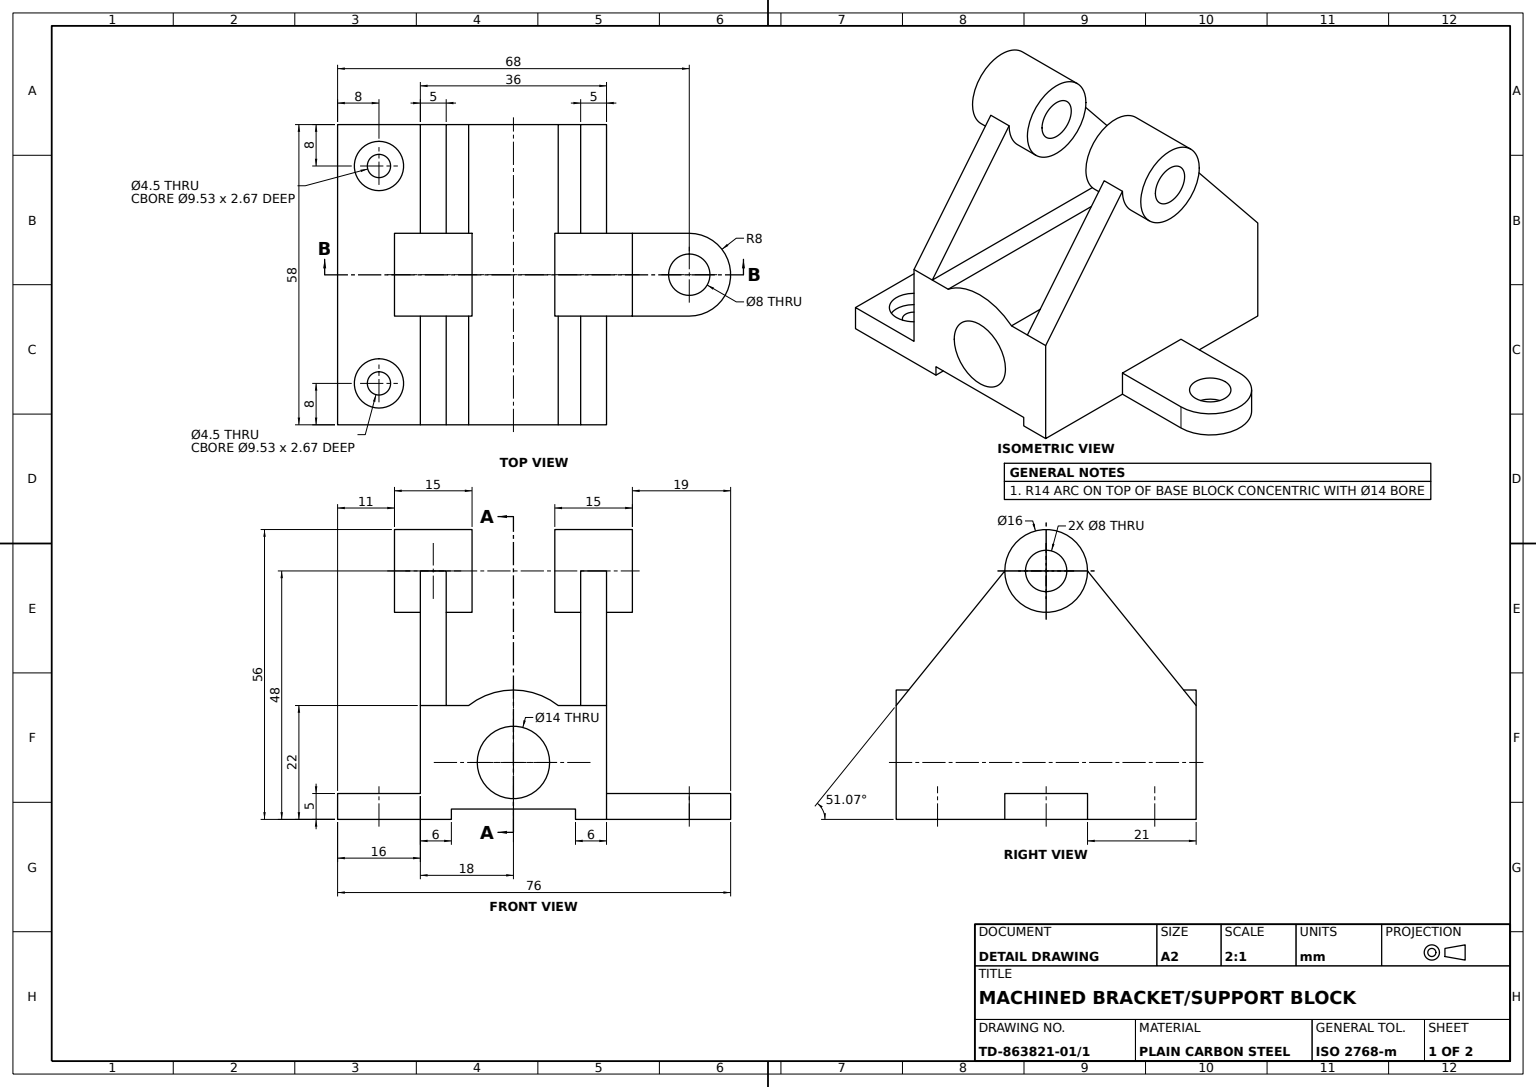
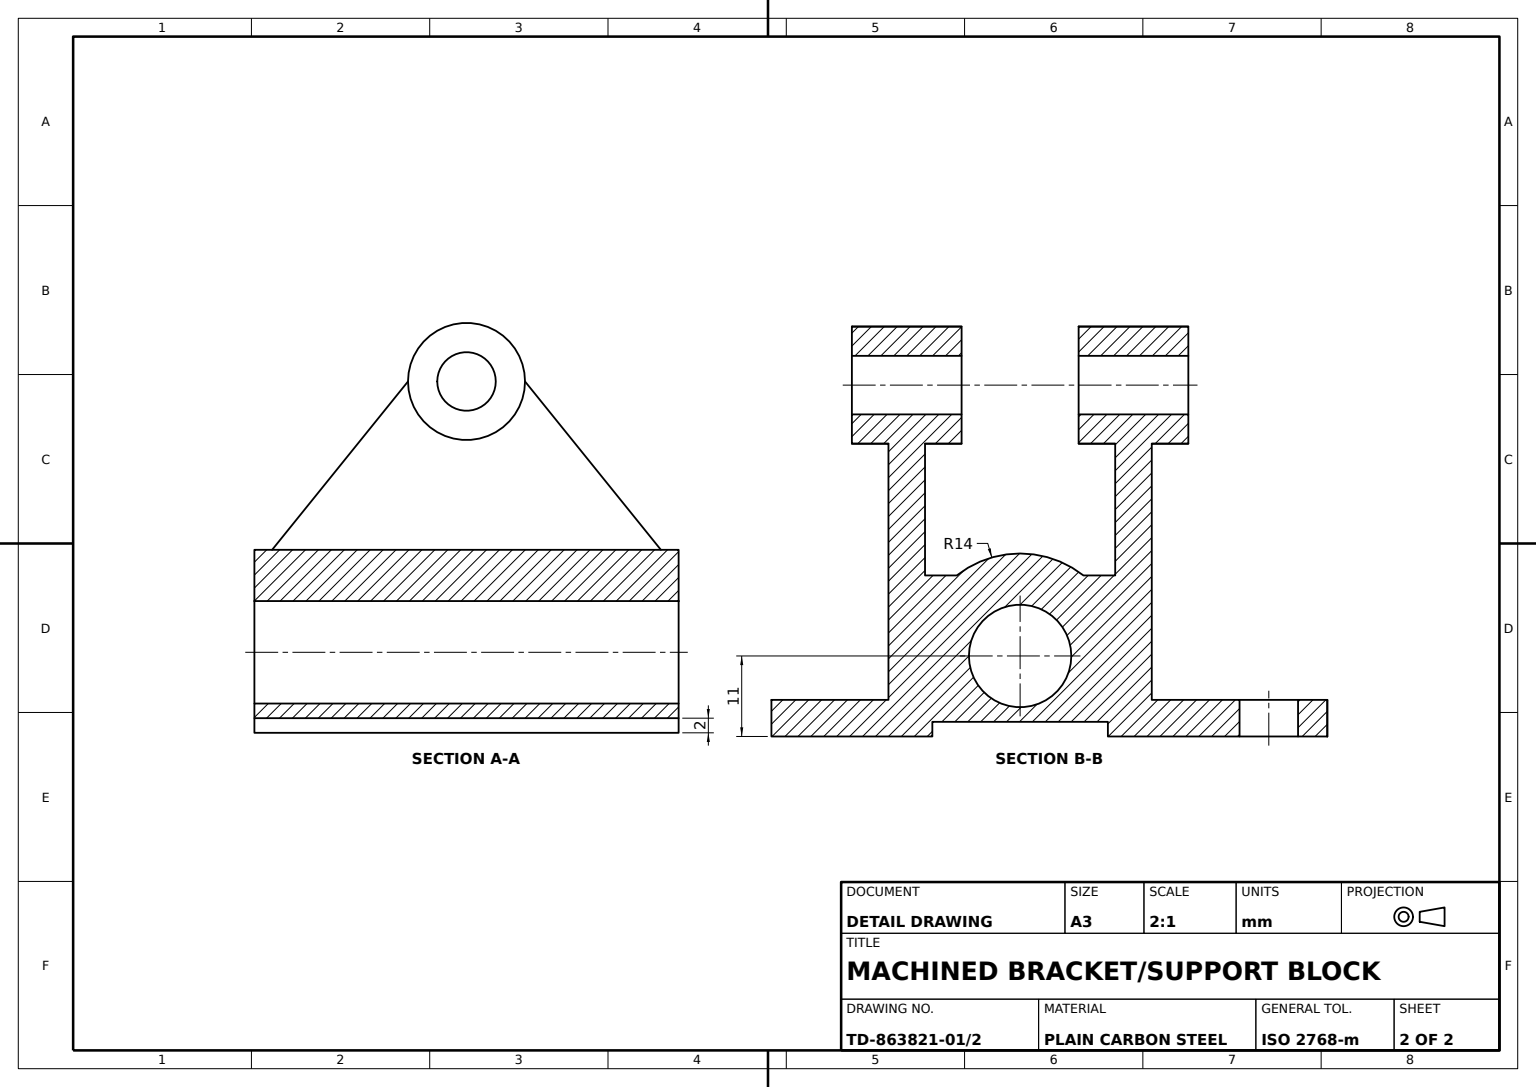
from build123d import *

# Parameters (mm, degrees)
BASE_BLOCK_DEPTH                = 58
FRONT_BORE_BOSS_DEPTH           = 58
FRONT_BORE_SKETCH_R             = 7
FRONT_BORE_DEPTH                = 73.698005475
LEFT_ARM_SKETCH_R               = 8
LEFT_ARM_SKETCH_R_2             = 4
LEFT_ARM_DEPTH                  = 5
LEFT_ARM_WEB_DEPTH              = 5
LEFT_START                      = 5
LEFT_PIVOT_BOSS_SKETCH_R        = 8
LEFT_PIVOT_BOSS_DEPTH           = 5
LEFT_PIVOT_HOLE_SKETCH_R        = 4
LEFT_PIVOT_HOLE_DEPTH           = 85.711274338
RIGHT_ARM_SKETCH_R              = 8
RIGHT_ARM_SKETCH_R_2            = 4
RIGHT_ARM_DEPTH                 = 5
RIGHT_ARM_WEB_DEPTH             = 5
RIGHT_PIVOT_BOSS_SKETCH_R       = 8
RIGHT_PIVOT_BOSS_DEPTH          = 5
RIGHT_PIVOT_HOLE_8_SKETCH_R     = 4
RIGHT_PIVOT_HOLE_8_DEPTH        = 87.377080293
SIDE_LUG_SKETCH_R               = 4
SIDE_LUG_DEPTH                  = 5
MOUNTING_TAB_SKETCH_W           = 16
MOUNTING_TAB_SKETCH_H           = 58
MOUNTING_TAB_DEPTH              = 5
M5_COUNTERBORE_HOLE_D           = 4.5
M5_COUNTERBORE_HOLE_CBORE_D     = 9.53
M5_COUNTERBORE_HOLE_CBORE_DEPTH = 2.67


with BuildPart() as part:
    # Base Block Profile → Base Block (new body)
    with BuildSketch(Plane.XY):
        Polygon((0, 0), (6, 0), (6, 2), (30, 2), (30, 0), (36, 0), (36, 22), (0, 22), align=None)
    extrude(amount=BASE_BLOCK_DEPTH)

    # Front Bore Boss Sketch → Front Bore Boss (add, through all)
    with BuildSketch(Plane.XY.offset(58)):
        with BuildLine():
            Line((4, 11), (32, 11))
            ThreePointArc((32, 11), (18, 25), (4, 11))
        make_face()
    extrude(amount=-FRONT_BORE_BOSS_DEPTH)

    # Front Bore Sketch → Front Bore (cut, through all)
    with BuildSketch(Plane.XY.offset(58)):
        with Locations((18, 11)):
            Circle(FRONT_BORE_SKETCH_R)
    extrude(amount=-FRONT_BORE_DEPTH, mode=Mode.SUBTRACT)



with BuildPart() as body_2:
    # Left Arm Sketch → Left Arm (new, symmetric)
    with BuildSketch(Plane(origin=(0, 0, 0), x_dir=(0, 0, -1), z_dir=(1, 0, 0))):
        with Locations((-29, 48)):
            Circle(LEFT_ARM_SKETCH_R)
        with Locations((-29, 48)):
            Circle(LEFT_ARM_SKETCH_R_2, mode=Mode.SUBTRACT)
    extrude(amount=LEFT_ARM_DEPTH, both=True)


with BuildPart() as part_1:
    add(part.part)

    add(body_2.part)  # Left Arm Web merges body 2
    # Left Arm Web Sketch → Left Arm Web (add)
    with BuildSketch(Plane(origin=(0, 0, 0), x_dir=(0, 0, -1), z_dir=(1, 0, 0))):
        with BuildLine():
            Line((-21, 48), (0, 22))
            Line((0, 22), (-58, 22))
            Line((-58, 22), (-37, 48))
            ThreePointArc((-37, 48), (-29, 40), (-21, 48))
        make_face()
    extrude(amount=LEFT_ARM_WEB_DEPTH)

    # Left Pivot Boss Sketch → Left Pivot Boss (add)
    with BuildSketch(Plane(origin=(5, 0, 0), x_dir=(0, 0, -1), z_dir=(1, 0, 0)).offset(LEFT_START)):
        with Locations((-29, 48)):
            Circle(LEFT_PIVOT_BOSS_SKETCH_R)
    extrude(amount=-LEFT_PIVOT_BOSS_DEPTH)

    # Left Pivot Hole Sketch → Left Pivot Hole (cut, through all)
    with BuildSketch(Plane(origin=(10, 0, 0), x_dir=(0, 0, -1), z_dir=(1, 0, 0))):
        with Locations((-29, 48)):
            Circle(LEFT_PIVOT_HOLE_SKETCH_R)
    extrude(amount=-LEFT_PIVOT_HOLE_DEPTH, mode=Mode.SUBTRACT)



with BuildPart() as body_2_2:
    # Right Arm Sketch → Right Arm (new, symmetric)
    with BuildSketch(Plane(origin=(36, 0, 0), x_dir=(0, 0, -1), z_dir=(1, 0, 0))):
        with Locations((-29, 48)):
            Circle(RIGHT_ARM_SKETCH_R)
        with Locations((-29, 48)):
            Circle(RIGHT_ARM_SKETCH_R_2, mode=Mode.SUBTRACT)
    extrude(amount=RIGHT_ARM_DEPTH, both=True)


with BuildPart() as part_2:
    add(part_1.part)

    add(body_2_2.part)  # Right Arm Web merges body 2 2
    # Right Arm Web Sketch → Right Arm Web (add)
    with BuildSketch(Plane(origin=(36, 0, 0), x_dir=(0, 0, -1), z_dir=(1, 0, 0))):
        with BuildLine():
            Line((-37, 48), (-58, 22))
            Line((-58, 22), (0, 22))
            Line((0, 22), (-21, 48))
            ThreePointArc((-21, 48), (-29, 40), (-37, 48))
        make_face()
    extrude(amount=-RIGHT_ARM_WEB_DEPTH)

    # Right Pivot Boss Sketch → Right Pivot Boss (add)
    with BuildSketch(Plane.ZY.offset(-31)):
        with Locations(Location((29, 48, 0), (0, 0, 180))):
            Circle(RIGHT_PIVOT_BOSS_SKETCH_R)
    extrude(amount=RIGHT_PIVOT_BOSS_DEPTH)

    # Right Pivot Hole Ø8 Sketch → Right Pivot Hole Ø8 (cut, through all)
    with BuildSketch(Plane.ZY.offset(-26)):
        with Locations(Location((29, 48, 0), (0, 0, 180))):
            Circle(RIGHT_PIVOT_HOLE_8_SKETCH_R)
    extrude(amount=-RIGHT_PIVOT_HOLE_8_DEPTH, mode=Mode.SUBTRACT)

    # Side Lug Sketch → Side Lug (add)
    with BuildSketch(Plane(origin=(0, 0, 0), x_dir=(1, 0, 0), z_dir=(0, 1, 0))):
        with BuildLine():
            Line((52, -21), (36, -21))
            Line((36, -21), (36, -37))
            Line((36, -37), (52, -37))
            ThreePointArc((52, -37), (60, -29), (52, -21))
        make_face()
        with Locations(Location((52, -29, 0), (0, 0, 270))):
            Circle(SIDE_LUG_SKETCH_R, mode=Mode.SUBTRACT)
    extrude(amount=SIDE_LUG_DEPTH)

    # Mounting Tab Sketch → Mounting Tab (add)
    with BuildSketch(Plane(origin=(0, 0, 0), x_dir=(1, 0, 0), z_dir=(0, 1, 0))):
        with Locations((-8, -29)):
            Rectangle(MOUNTING_TAB_SKETCH_W, MOUNTING_TAB_SKETCH_H)
    extrude(amount=MOUNTING_TAB_DEPTH)

    # M5 Counterbore Hole (through all)
    with Locations(Plane(origin=(0, 5, 0), x_dir=(1, 0, 0), z_dir=(0, 1, 0))):
        with Locations((-8, -8), (-8, -50)):
            CounterBoreHole(M5_COUNTERBORE_HOLE_D / 2, M5_COUNTERBORE_HOLE_CBORE_D / 2, M5_COUNTERBORE_HOLE_CBORE_DEPTH)


solid = part_2.part
